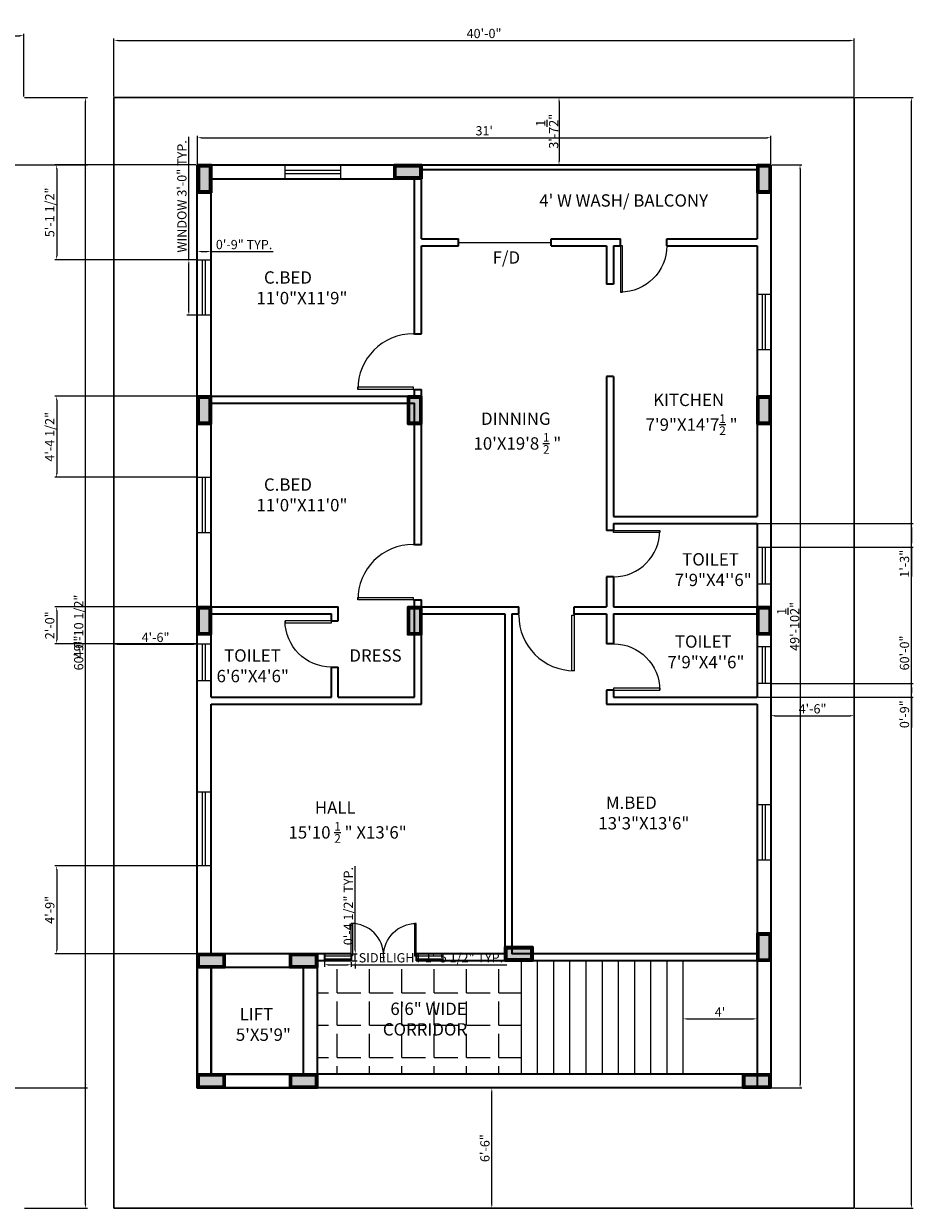
# Model space of a CAD drawing. Units: inches. Extents: x 1678 to 4856, y 4 to 3876.
# Tile 3 of 4: x 2753 to 3330, y 3108 to 3876. Entities that reach past the tile are written whole.
import ezdxf

# ---------------------------------------------------------------- set-up
doc = ezdxf.new("R2010")
doc.units = ezdxf.units.IN
for name, color, linetype, lineweight in [('A-ANNO-TEXT', 7, 'Continuous', 18), ('A-AREA-IDEN', 7, 'Continuous', 18), ('A-FLOR-EVTR', 7, 'Continuous', 35), ('A-FLOR-PATT', 252, 'Continuous', 13), ('COL', 6, 'Continuous', 40), ('compound wall', 7, 'Continuous', 30), ('DIMENSIONS', 6, 'Continuous', 18), ('doors', 2, 'Continuous', 18), ('stairs', 1, 'Continuous', 18), ('walls', 7, 'Continuous', 35), ('windows', 4, 'Continuous', 18)]:
    doc.layers.add(name, color=color, linetype=linetype, lineweight=lineweight)
doc.styles.get("Standard").update_dxf_attribs({"font": 'arial.ttf'})
doc.dimstyles.new('ISO-25', dxfattribs={"dimtxt": 6, "dimasz": 2.5, "dimexe": 1.25, "dimexo": 0.625, "dimtad": 1, "dimdec": 1, "dimlunit": 4, "dimtxsty": 'Standard', "dimcen": 2.5, "dimadec": 0, "dimazin": 0, "dimtfac": 1, "dimtdec": 1, "dimtmove": 0, "dimatfit": 3, "dimfxl": 1, "dimarcsym": 0})

# ---------------------------------------------------------------- blocks, each defined once
blk = doc.blocks.new('*U2')
for p, q in [((0, 0), (0, -6)), ((40, 0), (40, -6))]:
    blk.add_line(p, q)
blk.add_lwpolyline([(0, 0), (0, 40), (1.75, 40), (1.75, 0)], close=True)
blk.add_arc((0, 0), 40, 0, 90)
blk = doc.blocks.new('*D3')
at = {"layer": 'Defpoints', "color": 0, "transparency": 16777216}
for p in [(3180.72, 3232.03), (3228.72, 3232.03), (3228.72, 3231.08)]:
    blk.add_point(p, dxfattribs=at)
at = {"layer": 'DIMENSIONS', "color": 0, "lineweight": -2, "transparency": 16777216}
for p, q in [((3180.72, 3231.4), (3180.72, 3229.83)), ((3183.22, 3231.08), (3226.22, 3231.08)), ((3228.72, 3231.4), (3228.72, 3229.83))]:
    blk.add_line(p, q, dxfattribs=at)
at = {"layer": 'DIMENSIONS', "color": 0, "transparency": 16777216}
for points in [[(3183.22, 3231.5), (3183.22, 3230.67), (3180.72, 3231.08)], [(3226.22, 3231.5), (3226.22, 3230.67), (3228.72, 3231.08)]]:
    blk.add_solid(points, dxfattribs=at)
at = {"layer": 'DIMENSIONS', "color": 0, "transparency": 16777216, "insert": (3204.72, 3234.71), "char_height": 6, "attachment_point": 5}
blk.add_mtext("4'", dxfattribs=at)
blk = doc.blocks.new('*D4')
at = {"layer": 'Defpoints', "color": 0, "transparency": 16777216}
for p in [(3237.72, 3802.31), (2865.95, 3784.66), (3237.72, 3784.66)]:
    blk.add_point(p, dxfattribs=at)
at = {"layer": 'DIMENSIONS', "color": 0, "lineweight": -2, "transparency": 16777216}
for p, q in [((2865.95, 3785.29), (2865.95, 3803.56)), ((2868.45, 3802.31), (3235.22, 3802.31)), ((3237.72, 3785.29), (3237.72, 3803.56))]:
    blk.add_line(p, q, dxfattribs=at)
at = {"layer": 'DIMENSIONS', "color": 0, "transparency": 16777216}
for points in [[(2868.45, 3802.73), (2868.45, 3801.89), (2865.95, 3802.31)], [(3235.22, 3802.73), (3235.22, 3801.89), (3237.72, 3802.31)]]:
    blk.add_solid(points, dxfattribs=at)
at = {"layer": 'DIMENSIONS', "color": 0, "transparency": 16777216, "insert": (3051.84, 3806), "char_height": 6, "attachment_point": 5}
blk.add_mtext("31'", dxfattribs=at)
blk = doc.blocks.new('*D5')
at = {"layer": 'Defpoints', "color": 0, "transparency": 16777216}
for p in [(3083.8, 3828.28), (3083.8, 3784.66), (3100.35, 3784.66)]:
    blk.add_point(p, dxfattribs=at)
at = {"layer": 'DIMENSIONS', "color": 0, "lineweight": -2, "transparency": 16777216}
for p, q in [((3084.43, 3828.28), (3101.6, 3828.28)), ((3100.35, 3825.78), (3100.35, 3787.16)), ((3084.43, 3784.66), (3101.6, 3784.66))]:
    blk.add_line(p, q, dxfattribs=at)
at = {"layer": 'DIMENSIONS', "color": 0, "transparency": 16777216}
for points in [[(3099.93, 3825.78), (3100.76, 3825.78), (3100.35, 3828.28)], [(3099.93, 3787.16), (3100.76, 3787.16), (3100.35, 3784.66)]]:
    blk.add_solid(points, dxfattribs=at)
at = {"layer": 'DIMENSIONS', "color": 0, "transparency": 16777216, "insert": (3092.65, 3806.47), "char_height": 6, "attachment_point": 5, "rotation": 90}
blk.add_mtext('3\'-7{\\H1x;\\S1/2;}"', dxfattribs=at)
blk = doc.blocks.new('*D10')
at = {"layer": 'Defpoints', "color": 0, "transparency": 16777216}
for p in [(2865.72, 3473.89), (2811.72, 3468.28), (2865.72, 3468.28)]:
    blk.add_point(p, dxfattribs=at)
at = {"layer": 'DIMENSIONS', "color": 0, "lineweight": -2, "transparency": 16777216}
for p, q in [((2811.72, 3468.9), (2811.72, 3475.14)), ((2814.22, 3473.89), (2863.22, 3473.89)), ((2865.72, 3468.9), (2865.72, 3475.14))]:
    blk.add_line(p, q, dxfattribs=at)
at = {"layer": 'DIMENSIONS', "color": 0, "transparency": 16777216}
for points in [[(2814.22, 3474.31), (2814.22, 3473.47), (2811.72, 3473.89)], [(2863.22, 3474.31), (2863.22, 3473.47), (2865.72, 3473.89)]]:
    blk.add_solid(points, dxfattribs=at)
at = {"layer": 'DIMENSIONS', "color": 0, "transparency": 16777216, "insert": (2838.72, 3477.58), "char_height": 6, "attachment_point": 5}
blk.add_mtext('4\'-6"', dxfattribs=at)
blk = doc.blocks.new('*D11')
at = {"layer": 'Defpoints', "color": 0, "transparency": 16777216}
for p in [(3237.72, 3429.89), (3291.72, 3429.89), (3291.72, 3427.61)]:
    blk.add_point(p, dxfattribs=at)
at = {"layer": 'DIMENSIONS', "color": 0, "lineweight": -2, "transparency": 16777216}
for p, q in [((3237.72, 3429.27), (3237.72, 3426.36)), ((3240.22, 3427.61), (3289.22, 3427.61)), ((3291.72, 3429.27), (3291.72, 3426.36))]:
    blk.add_line(p, q, dxfattribs=at)
at = {"layer": 'DIMENSIONS', "color": 0, "transparency": 16777216}
for points in [[(3240.22, 3428.02), (3240.22, 3427.19), (3237.72, 3427.61)], [(3289.22, 3428.02), (3289.22, 3427.19), (3291.72, 3427.61)]]:
    blk.add_solid(points, dxfattribs=at)
at = {"layer": 'DIMENSIONS', "color": 0, "transparency": 16777216, "insert": (3264.72, 3431.29), "char_height": 6, "attachment_point": 5}
blk.add_mtext('4\'-6"', dxfattribs=at)
blk = doc.blocks.new('*D12')
at = {"layer": 'Defpoints', "color": 0, "transparency": 16777216}
for p in [(3034.26, 3186.28), (3056.74, 3186.28), (3034.26, 3108.28)]:
    blk.add_point(p, dxfattribs=at)
at = {"layer": 'DIMENSIONS', "color": 0, "lineweight": -2, "transparency": 16777216}
for p, q in [((3034.88, 3186.28), (3057.99, 3186.28)), ((3056.74, 3110.78), (3056.74, 3183.78)), ((3034.88, 3108.28), (3057.99, 3108.28))]:
    blk.add_line(p, q, dxfattribs=at)
at = {"layer": 'DIMENSIONS', "color": 0, "transparency": 16777216}
for points in [[(3056.33, 3183.78), (3057.16, 3183.78), (3056.74, 3186.28)], [(3056.33, 3110.78), (3057.16, 3110.78), (3056.74, 3108.28)]]:
    blk.add_solid(points, dxfattribs=at)
at = {"layer": 'DIMENSIONS', "color": 0, "transparency": 16777216, "insert": (3053.06, 3147.28), "char_height": 6, "attachment_point": 5, "rotation": 90}
blk.add_mtext('6\'-6"', dxfattribs=at)
blk = doc.blocks.new('*D16')
at = {"layer": 'Defpoints', "color": 0, "transparency": 16777216}
for p in [(3237.72, 3784.66), (3237.52, 3186.28), (3256.62, 3186.28)]:
    blk.add_point(p, dxfattribs=at)
at = {"layer": 'DIMENSIONS', "color": 0, "lineweight": -2, "transparency": 16777216}
for p, q in [((3238.34, 3784.66), (3257.87, 3784.66)), ((3256.62, 3782.16), (3256.62, 3188.78)), ((3238.15, 3186.28), (3257.87, 3186.28))]:
    blk.add_line(p, q, dxfattribs=at)
at = {"layer": 'DIMENSIONS', "color": 0, "transparency": 16777216}
for points in [[(3256.2, 3782.16), (3257.03, 3782.16), (3256.62, 3784.66)], [(3256.2, 3188.78), (3257.03, 3188.78), (3256.62, 3186.28)]]:
    blk.add_solid(points, dxfattribs=at)
at = {"layer": 'DIMENSIONS', "color": 0, "transparency": 16777216, "insert": (3248.92, 3485.47), "char_height": 6, "attachment_point": 5, "rotation": 90}
blk.add_mtext('49\'-10{\\H1x;\\S1/2;}"', dxfattribs=at)
blk = doc.blocks.new('COLUMN-9x18')
h = blk.add_hatch(color=256)
h.dxf.hatch_style = 1
h.paths.add_polyline_path([(8, 1), (8, 17), (1, 17), (1, 1)])
for points in [[(9, 18), (9, 0), (0, 0), (0, 18)], [(8, 17), (8, 1), (1, 1), (1, 17)]]:
    blk.add_lwpolyline(points, close=True)
blk = doc.blocks.new('WIN-36')
for p, q in [((3.5, 0), (3.5, 36)), ((5.5, 0), (5.5, 36))]:
    blk.add_line(p, q)
blk.add_lwpolyline([(0, 0), (0, 36), (9, 36), (9, 0)], close=True)
blk = doc.blocks.new('WIN-24')
for p, q in [((3.5, 0), (3.5, 24)), ((5.5, 0), (5.5, 24))]:
    blk.add_line(p, q)
blk.add_lwpolyline([(0, 0), (0, 24), (9, 24), (9, 0)], close=True)
blk = doc.blocks.new('WIN-48')
for p, q in [((3.5, 0), (3.5, 48)), ((5.5, 0), (5.5, 48))]:
    blk.add_line(p, q)
blk.add_lwpolyline([(0, 0), (0, 48), (9, 48), (9, 0)], close=True)
blk = doc.blocks.new('WIN-ENTRY-SIDELIGHT')
for p, q in [((0, 3.25), (17.39, 3.25)), ((0, 1.25), (17.39, 1.25))]:
    blk.add_line(p, q)
blk.add_lwpolyline([(0, 4.5), (17.39, 4.5), (17.39, 0), (0, 0)], close=True)
blk = doc.blocks.new('SITE-PERIMETER-40x60')
for p, q in [((0, 720), (480, 720)), ((0, 0), (0, 720)), ((480, 720), (480, 0)), ((480, 0), (0, 0))]:
    blk.add_line(p, q)
blk = doc.blocks.new('STAIR-FLIGHT-11-TREAD-LINES')
for p, q in [((0, 73.5), (0, 0)), ((10.5, 73.5), (10.5, 0)), ((21, 73.5), (21, 0)), ((31.5, 73.5), (31.5, 0)), ((42, 73.5), (42, 0)), ((52.5, 73.5), (52.5, 0)), ((63, 73.5), (63, 0)), ((73.5, 73.5), (73.5, 0)), ((84, 73.5), (84, 0)), ((94.5, 73.5), (94.5, 0)), ((105, 73.5), (105, 0))]:
    blk.add_line(p, q)
blk = doc.blocks.new('LIFT-SHAFT-60x69')
for p, q in [((9, 9), (9, 78)), ((69, 9), (9, 9))]:
    blk.add_line(p, q)
blk.add_lwpolyline([(78, 87), (78, 87), (0, 87), (0, 0), (78, 0), (78, 82.5)])
blk.add_lwpolyline([(9, 9), (69, 9), (69, 78), (9, 78)], close=True)
blk = doc.blocks.new('*D48')
at = {"layer": 'Defpoints', "color": 0, "transparency": 16777216}
for p in [(2860.32, 3723.16), (2865.72, 3723.16), (2865.72, 3687.16)]:
    blk.add_point(p, dxfattribs=at)
at = {"layer": 'DIMENSIONS', "color": 0, "lineweight": -2, "transparency": 16777216}
for p, q in [((2860.32, 3723.16), (2860.32, 3802.84)), ((2865.09, 3723.16), (2859.07, 3723.16)), ((2860.32, 3689.66), (2860.32, 3720.66)), ((2865.09, 3687.16), (2859.07, 3687.16))]:
    blk.add_line(p, q, dxfattribs=at)
at = {"layer": 'DIMENSIONS', "color": 0, "transparency": 16777216}
for points in [[(2859.9, 3720.66), (2860.73, 3720.66), (2860.32, 3723.16)], [(2859.9, 3689.66), (2860.73, 3689.66), (2860.32, 3687.16)]]:
    blk.add_solid(points, dxfattribs=at)
at = {"layer": 'DIMENSIONS', "color": 0, "transparency": 16777216, "insert": (2856.59, 3764.25), "char_height": 6, "attachment_point": 5, "rotation": 90}
blk.add_mtext('WINDOW 3\'-0" TYP.', dxfattribs=at)
blk = doc.blocks.new('*D49')
at = {"layer": 'Defpoints', "color": 0, "transparency": 16777216}
for p in [(2874.72, 3728.56), (2865.72, 3723.16), (2874.72, 3723.16)]:
    blk.add_point(p, dxfattribs=at)
at = {"layer": 'DIMENSIONS', "color": 0, "lineweight": -2, "transparency": 16777216}
for p, q in [((2865.72, 3723.79), (2865.72, 3729.81)), ((2868.22, 3728.56), (2872.22, 3728.56)), ((2874.72, 3723.79), (2874.72, 3729.81)), ((2874.72, 3728.56), (2915.04, 3728.56))]:
    blk.add_line(p, q, dxfattribs=at)
at = {"layer": 'DIMENSIONS', "color": 0, "transparency": 16777216}
for points in [[(2868.22, 3728.98), (2868.22, 3728.15), (2865.72, 3728.56)], [(2872.22, 3728.98), (2872.22, 3728.15), (2874.72, 3728.56)]]:
    blk.add_solid(points, dxfattribs=at)
at = {"layer": 'DIMENSIONS', "color": 0, "transparency": 16777216, "insert": (2896.13, 3732.25), "char_height": 6, "attachment_point": 5}
blk.add_mtext('0\'-9" TYP.', dxfattribs=at)
blk = doc.blocks.new('*D54')
at = {"layer": 'Defpoints', "color": 0, "transparency": 16777216}
for p in [(2948.22, 3268.78), (2965.61, 3268.78), (2965.61, 3266.17)]:
    blk.add_point(p, dxfattribs=at)
at = {"layer": 'DIMENSIONS', "color": 0, "lineweight": -2, "transparency": 16777216}
for p, q in [((2948.22, 3268.15), (2948.22, 3264.92)), ((2950.72, 3266.17), (2963.11, 3266.17)), ((2965.61, 3268.15), (2965.61, 3264.92)), ((2965.61, 3266.17), (3066.46, 3266.17))]:
    blk.add_line(p, q, dxfattribs=at)
at = {"layer": 'DIMENSIONS', "color": 0, "transparency": 16777216}
for points in [[(2950.72, 3266.59), (2950.72, 3265.75), (2948.22, 3266.17)], [(2963.11, 3266.59), (2963.11, 3265.75), (2965.61, 3266.17)]]:
    blk.add_solid(points, dxfattribs=at)
at = {"layer": 'DIMENSIONS', "color": 0, "transparency": 16777216, "insert": (3017.28, 3269.9), "char_height": 6, "attachment_point": 5}
blk.add_mtext('SIDELIGHT 1\'-5 1/2" TYP.', dxfattribs=at)
blk = doc.blocks.new('*D55')
at = {"layer": 'Defpoints', "color": 0, "transparency": 16777216}
for p in [(2965.61, 3273.28), (2968.22, 3273.28), (2965.61, 3268.78)]:
    blk.add_point(p, dxfattribs=at)
at = {"layer": 'DIMENSIONS', "color": 0, "lineweight": -2, "transparency": 16777216}
for p, q in [((2968.22, 3275.78), (2968.22, 3330.08)), ((2966.23, 3273.28), (2969.47, 3273.28)), ((2968.22, 3268.78), (2968.22, 3273.28)), ((2966.23, 3268.78), (2969.47, 3268.78)), ((2968.22, 3266.28), (2968.22, 3263.78))]:
    blk.add_line(p, q, dxfattribs=at)
at = {"layer": 'DIMENSIONS', "color": 0, "transparency": 16777216}
for points in [[(2967.8, 3275.78), (2968.63, 3275.78), (2968.22, 3273.28)], [(2967.8, 3266.28), (2968.63, 3266.28), (2968.22, 3268.78)]]:
    blk.add_solid(points, dxfattribs=at)
at = {"layer": 'DIMENSIONS', "color": 0, "transparency": 16777216, "insert": (2964.49, 3304.18), "char_height": 6, "attachment_point": 5, "rotation": 90}
blk.add_mtext('0\'-4 1/2" TYP.', dxfattribs=at)
blk = doc.blocks.new('*D57')
at = {"layer": 'Defpoints', "color": 0, "transparency": 16777216}
for p in [(2753.23, 3868.43), (2273.23, 3828.28), (2753.23, 3828.28)]:
    blk.add_point(p, dxfattribs=at)
at = {"layer": 'DIMENSIONS', "color": 0, "lineweight": -2, "transparency": 16777216}
for p, q in [((2273.23, 3828.9), (2273.23, 3869.68)), ((2275.73, 3868.43), (2750.73, 3868.43)), ((2753.23, 3828.9), (2753.23, 3869.68))]:
    blk.add_line(p, q, dxfattribs=at)
at = {"layer": 'DIMENSIONS', "color": 0, "transparency": 16777216}
for points in [[(2275.73, 3868.84), (2275.73, 3868.01), (2273.23, 3868.43)], [(2750.73, 3868.84), (2750.73, 3868.01), (2753.23, 3868.43)]]:
    blk.add_solid(points, dxfattribs=at)
at = {"layer": 'DIMENSIONS', "color": 0, "transparency": 16777216, "insert": (2513.23, 3872.12), "char_height": 6, "attachment_point": 5}
blk.add_mtext('40\'-0"', dxfattribs=at)
blk = doc.blocks.new('*D58')
at = {"layer": 'Defpoints', "color": 0, "transparency": 16777216}
for p in [(2753.23, 3828.28), (2793.38, 3828.28), (2753.23, 3108.28)]:
    blk.add_point(p, dxfattribs=at)
at = {"layer": 'DIMENSIONS', "color": 0, "lineweight": -2, "transparency": 16777216}
for p, q in [((2753.85, 3828.28), (2794.63, 3828.28)), ((2793.38, 3110.78), (2793.38, 3825.78)), ((2753.85, 3108.28), (2794.63, 3108.28))]:
    blk.add_line(p, q, dxfattribs=at)
at = {"layer": 'DIMENSIONS', "color": 0, "transparency": 16777216}
for points in [[(2792.96, 3825.78), (2793.8, 3825.78), (2793.38, 3828.28)], [(2792.96, 3110.78), (2793.8, 3110.78), (2793.38, 3108.28)]]:
    blk.add_solid(points, dxfattribs=at)
at = {"layer": 'DIMENSIONS', "color": 0, "transparency": 16777216, "insert": (2789.69, 3468.28), "char_height": 6, "attachment_point": 5, "rotation": 90}
blk.add_mtext('60\'-0"', dxfattribs=at)
blk = doc.blocks.new('*D59')
at = {"layer": 'Defpoints', "color": 0, "transparency": 16777216}
for p in [(2699.23, 3784.66), (2793.38, 3784.66), (2699.23, 3186.28)]:
    blk.add_point(p, dxfattribs=at)
at = {"layer": 'DIMENSIONS', "color": 0, "lineweight": -2, "transparency": 16777216}
for p, q in [((2699.85, 3784.66), (2794.63, 3784.66)), ((2793.38, 3188.78), (2793.38, 3782.16)), ((2699.85, 3186.28), (2794.63, 3186.28))]:
    blk.add_line(p, q, dxfattribs=at)
at = {"layer": 'DIMENSIONS', "color": 0, "transparency": 16777216}
for points in [[(2792.96, 3782.16), (2793.8, 3782.16), (2793.38, 3784.66)], [(2792.96, 3188.78), (2793.8, 3188.78), (2793.38, 3186.28)]]:
    blk.add_solid(points, dxfattribs=at)
at = {"layer": 'DIMENSIONS', "color": 0, "transparency": 16777216, "insert": (2789.65, 3485.47), "char_height": 6, "attachment_point": 5, "rotation": 90}
blk.add_mtext('49\'-10 1/2"', dxfattribs=at)
blk = doc.blocks.new('*D61')
at = {"layer": 'Defpoints', "color": 0, "transparency": 16777216}
for p in [(3291.72, 3865.38), (2811.72, 3828.28), (3291.72, 3828.28)]:
    blk.add_point(p, dxfattribs=at)
at = {"layer": 'DIMENSIONS', "color": 0, "lineweight": -2, "transparency": 16777216}
for p, q in [((2811.72, 3828.9), (2811.72, 3866.63)), ((2814.22, 3865.38), (3289.22, 3865.38)), ((3291.72, 3828.9), (3291.72, 3866.63))]:
    blk.add_line(p, q, dxfattribs=at)
at = {"layer": 'DIMENSIONS', "color": 0, "transparency": 16777216}
for points in [[(2814.22, 3865.79), (2814.22, 3864.96), (2811.72, 3865.38)], [(3289.22, 3865.79), (3289.22, 3864.96), (3291.72, 3865.38)]]:
    blk.add_solid(points, dxfattribs=at)
at = {"layer": 'DIMENSIONS', "color": 0, "transparency": 16777216, "insert": (3051.72, 3869.07), "char_height": 6, "attachment_point": 5}
blk.add_mtext('40\'-0"', dxfattribs=at)
blk = doc.blocks.new('*D76')
at = {"layer": 'Defpoints', "color": 0, "transparency": 16777216}
for p in [(2865.72, 3784.66), (2774.62, 3723.16), (2865.72, 3723.16)]:
    blk.add_point(p, dxfattribs=at)
at = {"layer": 'DIMENSIONS', "color": 0, "lineweight": -2, "transparency": 16777216}
for p, q in [((2865.09, 3784.66), (2773.37, 3784.66)), ((2774.62, 3782.16), (2774.62, 3725.66)), ((2865.09, 3723.16), (2773.37, 3723.16))]:
    blk.add_line(p, q, dxfattribs=at)
at = {"layer": 'DIMENSIONS', "color": 0, "transparency": 16777216}
for points in [[(2774.2, 3782.16), (2775.03, 3782.16), (2774.62, 3784.66)], [(2774.2, 3725.66), (2775.03, 3725.66), (2774.62, 3723.16)]]:
    blk.add_solid(points, dxfattribs=at)
at = {"layer": 'DIMENSIONS', "color": 0, "transparency": 16777216, "insert": (2770.89, 3753.91), "char_height": 6, "attachment_point": 5, "rotation": 90}
blk.add_mtext('5\'-1 1/2"', dxfattribs=at)
blk = doc.blocks.new('*D77')
at = {"layer": 'Defpoints', "color": 0, "transparency": 16777216}
for p in [(2865.72, 3634.66), (2774.62, 3582.16), (2865.72, 3582.16)]:
    blk.add_point(p, dxfattribs=at)
at = {"layer": 'DIMENSIONS', "color": 0, "lineweight": -2, "transparency": 16777216}
for p, q in [((2865.09, 3634.66), (2773.37, 3634.66)), ((2774.62, 3632.16), (2774.62, 3584.66)), ((2865.09, 3582.16), (2773.37, 3582.16))]:
    blk.add_line(p, q, dxfattribs=at)
at = {"layer": 'DIMENSIONS', "color": 0, "transparency": 16777216}
for points in [[(2774.2, 3632.16), (2775.03, 3632.16), (2774.62, 3634.66)], [(2774.2, 3584.66), (2775.03, 3584.66), (2774.62, 3582.16)]]:
    blk.add_solid(points, dxfattribs=at)
at = {"layer": 'DIMENSIONS', "color": 0, "transparency": 16777216, "insert": (2770.89, 3608.41), "char_height": 6, "attachment_point": 5, "rotation": 90}
blk.add_mtext('4\'-4 1/2"', dxfattribs=at)
blk = doc.blocks.new('*D78')
at = {"layer": 'Defpoints', "color": 0, "transparency": 16777216}
for p in [(2865.72, 3498.16), (2774.62, 3474.26), (2865.72, 3474.26)]:
    blk.add_point(p, dxfattribs=at)
at = {"layer": 'DIMENSIONS', "color": 0, "lineweight": -2, "transparency": 16777216}
for p, q in [((2865.09, 3498.16), (2773.37, 3498.16)), ((2774.62, 3495.66), (2774.62, 3476.76)), ((2865.09, 3474.26), (2773.37, 3474.26))]:
    blk.add_line(p, q, dxfattribs=at)
at = {"layer": 'DIMENSIONS', "color": 0, "transparency": 16777216}
for points in [[(2774.2, 3495.66), (2775.03, 3495.66), (2774.62, 3498.16)], [(2774.2, 3476.76), (2775.03, 3476.76), (2774.62, 3474.26)]]:
    blk.add_solid(points, dxfattribs=at)
at = {"layer": 'DIMENSIONS', "color": 0, "transparency": 16777216, "insert": (2770.93, 3486.21), "char_height": 6, "attachment_point": 5, "rotation": 90}
blk.add_mtext('2\'-0"', dxfattribs=at)
blk = doc.blocks.new('*D79')
at = {"layer": 'Defpoints', "color": 0, "transparency": 16777216}
for p in [(2865.72, 3330.22), (2774.62, 3273.28), (2865.72, 3273.28)]:
    blk.add_point(p, dxfattribs=at)
at = {"layer": 'DIMENSIONS', "color": 0, "lineweight": -2, "transparency": 16777216}
for p, q in [((2865.09, 3330.22), (2773.37, 3330.22)), ((2774.62, 3327.72), (2774.62, 3275.78)), ((2865.09, 3273.28), (2773.37, 3273.28))]:
    blk.add_line(p, q, dxfattribs=at)
at = {"layer": 'DIMENSIONS', "color": 0, "transparency": 16777216}
for points in [[(2774.2, 3327.72), (2775.03, 3327.72), (2774.62, 3330.22)], [(2774.2, 3275.78), (2775.03, 3275.78), (2774.62, 3273.28)]]:
    blk.add_solid(points, dxfattribs=at)
at = {"layer": 'DIMENSIONS', "color": 0, "transparency": 16777216, "insert": (2770.93, 3301.75), "char_height": 6, "attachment_point": 5, "rotation": 90}
blk.add_mtext('4\'-9"', dxfattribs=at)
blk = doc.blocks.new('*D85')
at = {"layer": 'Defpoints', "color": 0, "transparency": 16777216}
for p in [(3228.72, 3552.16), (3237.72, 3536.94), (3328.82, 3536.94)]:
    blk.add_point(p, dxfattribs=at)
at = {"layer": 'DIMENSIONS', "color": 0, "lineweight": -2, "transparency": 16777216}
for p, q in [((3229.34, 3552.16), (3330.07, 3552.16)), ((3328.82, 3549.66), (3328.82, 3539.44)), ((3238.34, 3536.94), (3330.07, 3536.94)), ((3328.82, 3536.94), (3328.82, 3517.81))]:
    blk.add_line(p, q, dxfattribs=at)
at = {"layer": 'DIMENSIONS', "color": 0, "transparency": 16777216}
for points in [[(3328.4, 3549.66), (3329.23, 3549.66), (3328.82, 3552.16)], [(3328.4, 3539.44), (3329.23, 3539.44), (3328.82, 3536.94)]]:
    blk.add_solid(points, dxfattribs=at)
at = {"layer": 'DIMENSIONS', "color": 0, "transparency": 16777216, "insert": (3325.13, 3526.12), "char_height": 6, "attachment_point": 5, "rotation": 90}
blk.add_mtext('1\'-3"', dxfattribs=at)
blk = doc.blocks.new('*D86')
at = {"layer": 'Defpoints', "color": 0, "transparency": 16777216}
for p in [(3237.72, 3448.44), (3228.72, 3439.66), (3328.82, 3439.66)]:
    blk.add_point(p, dxfattribs=at)
at = {"layer": 'DIMENSIONS', "color": 0, "lineweight": -2, "transparency": 16777216}
for p, q in [((3238.34, 3448.44), (3330.07, 3448.44)), ((3328.82, 3445.94), (3328.82, 3442.16)), ((3229.34, 3439.66), (3330.07, 3439.66)), ((3328.82, 3439.66), (3328.82, 3419.96))]:
    blk.add_line(p, q, dxfattribs=at)
at = {"layer": 'DIMENSIONS', "color": 0, "transparency": 16777216}
for points in [[(3328.4, 3445.94), (3329.23, 3445.94), (3328.82, 3448.44)], [(3328.4, 3442.16), (3329.23, 3442.16), (3328.82, 3439.66)]]:
    blk.add_solid(points, dxfattribs=at)
at = {"layer": 'DIMENSIONS', "color": 0, "transparency": 16777216, "insert": (3325.13, 3428.56), "char_height": 6, "attachment_point": 5, "rotation": 90}
blk.add_mtext('0\'-9"', dxfattribs=at)
blk = doc.blocks.new('*D87')
at = {"layer": 'Defpoints', "color": 0, "transparency": 16777216}
for p in [(3291.72, 3828.28), (3328.82, 3828.28), (3291.72, 3108.28)]:
    blk.add_point(p, dxfattribs=at)
at = {"layer": 'DIMENSIONS', "color": 0, "lineweight": -2, "transparency": 16777216}
for p, q in [((3292.34, 3828.28), (3330.07, 3828.28)), ((3328.82, 3110.78), (3328.82, 3825.78)), ((3292.34, 3108.28), (3330.07, 3108.28))]:
    blk.add_line(p, q, dxfattribs=at)
at = {"layer": 'DIMENSIONS', "color": 0, "transparency": 16777216}
for points in [[(3328.4, 3825.78), (3329.23, 3825.78), (3328.82, 3828.28)], [(3328.4, 3110.78), (3329.23, 3110.78), (3328.82, 3108.28)]]:
    blk.add_solid(points, dxfattribs=at)
at = {"layer": 'DIMENSIONS', "color": 0, "transparency": 16777216, "insert": (3325.13, 3468.28), "char_height": 6, "attachment_point": 5, "rotation": 90}
blk.add_mtext('60\'-0"', dxfattribs=at)

msp = doc.modelspace()

# ---------------------------------------------------------------- hatches: boundary and pattern name
at = {"layer": 'A-FLOR-PATT'}
h = msp.add_hatch(dxfattribs=at)
h.set_pattern_fill('ANGLE', color=256, scale=3)
h.set_pattern_definition([(0, (1238.245, 0), (0, 20.955), [15.24, -5.715]), (90, (1238.245, 0), (-20.955, 1e-15), [15.24, -5.715])])
h.paths.add_polyline_path([(3075.72, 3268.78), (2943.72, 3268.78), (2943.72, 3195.28), (3075.72, 3195.28)])

# ---------------------------------------------------------------- linework, layer by layer
at = {"layer": 'doors'}
msp.add_line((3035.22, 3734.41), (3095.22, 3734.41), dxfattribs=at)
at = {"layer": 'walls'}
for p, q in [((2865.72, 3784.66), (3237.72, 3784.66)), ((2865.72, 3186.28), (2865.72, 3784.66)), ((3011.22, 3781.66), (3228.72, 3781.66)), ((3011.22, 3736.66), (3011.22, 3781.66)), ((3228.72, 3781.66), (3228.72, 3736.66)), ((3237.72, 3784.66), (3237.72, 3186.28)), ((2874.72, 3775.66), (3006.72, 3775.66)), ((2874.72, 3634.66), (2874.72, 3775.66)), ((3006.72, 3675.16), (3006.72, 3775.66)), ((3011.22, 3736.66), (3035.22, 3736.66)), ((3011.22, 3732.16), (3035.22, 3732.16)), ((3011.22, 3675.16), (3011.22, 3732.16)), ((3035.22, 3732.16), (3035.22, 3736.66)), ((3095.22, 3732.16), (3095.22, 3736.66)), ((3095.22, 3736.66), (3140.22, 3736.66)), ((3095.22, 3732.16), (3131.22, 3732.16)), ((3131.22, 3732.16), (3131.22, 3707.41)), ((3135.72, 3732.16), (3135.72, 3707.41)), ((3135.72, 3732.16), (3140.22, 3732.16)), ((3140.22, 3732.16), (3140.22, 3736.66)), ((3170.22, 3732.16), (3170.22, 3736.66)), ((3170.22, 3736.66), (3228.72, 3736.66)), ((3170.22, 3732.16), (3228.72, 3732.16)), ((3228.72, 3732.16), (3228.72, 3556.66)), ((3135.72, 3707.41), (3131.22, 3707.41)), ((3006.72, 3675.16), (3011.22, 3675.16)), ((3135.72, 3647.41), (3131.22, 3647.41)), ((3131.22, 3647.41), (3131.22, 3547.66)), ((3135.72, 3647.41), (3135.72, 3556.66)), ((2874.72, 3634.66), (3006.72, 3634.66)), ((3006.72, 3634.66), (3006.72, 3639.16)), ((3006.72, 3639.16), (3011.22, 3639.16)), ((3011.22, 3538.66), (3011.22, 3639.16)), ((2874.72, 3630.16), (3006.72, 3630.16)), ((2874.72, 3498.16), (2874.72, 3630.16)), ((3006.72, 3538.66), (3006.72, 3630.16)), ((3135.72, 3630.16), (3135.72, 3556.66)), ((3135.72, 3556.66), (3228.72, 3556.66)), ((3135.72, 3552.16), (3228.72, 3552.16)), ((3135.72, 3552.16), (3135.72, 3547.66)), ((3228.72, 3552.16), (3228.72, 3498.16)), ((3135.72, 3547.66), (3131.22, 3547.66)), ((3006.72, 3538.66), (3011.22, 3538.66)), ((3135.72, 3517.66), (3131.22, 3517.66)), ((3131.22, 3517.66), (3131.22, 3498.16)), ((3135.72, 3517.66), (3135.72, 3498.16)), ((3006.72, 3498.16), (3006.72, 3502.66)), ((3006.72, 3502.66), (3011.22, 3502.66)), ((3011.22, 3498.16), (3011.22, 3502.66)), ((2874.72, 3498.16), (2957.22, 3498.16)), ((2957.22, 3489.16), (2957.22, 3498.16)), ((3006.72, 3439.66), (3006.72, 3498.16)), ((3011.22, 3498.16), (3074.22, 3498.16)), ((3074.22, 3493.66), (3074.22, 3498.16)), ((3110.22, 3493.66), (3110.22, 3498.16)), ((3110.22, 3498.16), (3131.22, 3498.16)), ((3135.72, 3498.16), (3228.72, 3498.16)), ((2874.72, 3493.66), (2952.72, 3493.66)), ((2874.72, 3439.66), (2874.72, 3493.66)), ((2952.72, 3489.16), (2952.72, 3493.66)), ((2952.72, 3489.16), (2957.22, 3489.16)), ((2957.22, 3489.16), (2957.22, 3489.16)), ((3011.22, 3435.16), (3011.22, 3493.66)), ((3011.22, 3493.66), (3065.22, 3493.66)), ((3065.22, 3493.66), (3065.22, 3273.28)), ((3069.72, 3493.66), (3069.72, 3273.28)), ((3069.72, 3493.66), (3074.22, 3493.66)), ((3110.22, 3493.66), (3131.22, 3493.66)), ((3131.22, 3493.66), (3131.22, 3474.16)), ((3135.72, 3493.66), (3228.72, 3493.66)), ((3135.72, 3493.66), (3135.72, 3474.16)), ((3228.72, 3493.66), (3228.72, 3439.66)), ((3135.72, 3474.16), (3131.22, 3474.16)), ((2952.72, 3439.66), (2952.72, 3459.16)), ((2952.72, 3459.16), (2957.22, 3459.16)), ((2957.22, 3439.66), (2957.22, 3459.16)), ((3135.72, 3444.16), (3131.22, 3444.16)), ((3131.22, 3444.16), (3131.22, 3435.16)), ((3135.72, 3444.16), (3135.72, 3439.66)), ((2874.72, 3439.66), (2952.72, 3439.66)), ((2874.72, 3435.16), (3011.22, 3435.16)), ((2874.72, 3273.28), (2874.72, 3435.16)), ((2957.22, 3439.66), (3006.72, 3439.66)), ((3131.22, 3435.16), (3228.72, 3435.16)), ((3135.72, 3439.66), (3228.72, 3439.66)), ((3228.72, 3435.16), (3228.72, 3268.78)), ((2965.61, 3273.28), (2874.72, 3273.28)), ((2948.22, 3273.28), (2948.22, 3268.78)), ((2948.22, 3273.28), (2948.22, 3268.78)), ((2965.61, 3273.28), (2965.61, 3268.78)), ((3065.22, 3273.28), (3007.61, 3273.28)), ((3007.61, 3273.28), (3007.61, 3268.78)), ((3228.72, 3273.28), (3069.72, 3273.28)), ((2965.61, 3268.78), (2943.72, 3268.78)), ((3228.72, 3268.78), (3007.61, 3268.78)), ((3228.72, 3268.78), (3228.72, 3186.28)), ((3237.72, 3195.28), (2943.72, 3195.28)), ((3237.72, 3186.28), (2865.72, 3186.28))]:
    msp.add_line(p, q, dxfattribs=at)

# ---------------------------------------------------------------- block references
at = {"layer": 'A-FLOR-EVTR'}
msp.add_blockref('LIFT-SHAFT-60x69', (2865.72, 3186.28), dxfattribs=at)
at = {"layer": 'COL'}
for p in [(2865.95, 3766.66), (3228.72, 3766.66), (2865.72, 3616.66), (3002.22, 3616.69), (3228.72, 3616.69), (2865.72, 3480.16), (3002.22, 3480.16), (3228.72, 3480.16), (3228.72, 3268.61)]:
    msp.add_blockref('COLUMN-9x18', p, dxfattribs=at)
for p, rotation in [((3011.35, 3775.66), 90.0000000000118), ((2883.72, 3264.28), 90.00000000000551), ((2943.72, 3264.28), 90.00000000000551), ((3083.27, 3268.78), 90.0000000000076), ((2883.72, 3186.28), 90.00000000000551), ((2943.72, 3186.28), 90.00000000000551), ((3237.52, 3186.28), 90.0000000000076)]:
    msp.add_blockref('COLUMN-9x18', p, dxfattribs=dict(at, rotation=rotation))
at = {"layer": 'compound wall', "rotation": 180}
msp.add_blockref('SITE-PERIMETER-40x60', (3291.72, 3828.28), dxfattribs=at)
at = {"layer": 'doors'}
for p, xscale, yscale, zscale, rotation in [((3140.22, 3732.16), -0.75, 0.75, 0.75, 180), ((3005.82, 3639.16), 0.9, 0.9, 0.9, 89.99999999999999), ((3135.72, 3547.66), 0.75, 0.75, 0.75, 270), ((3005.82, 3502.66), 0.9, 0.9, 0.9, 89.99999999999999), ((3110.22, 3492.76), 0.9, 0.9, 0.9, 180), ((2952.72, 3489.16), -0.75, 0.75, 0.75, 90), ((3135.72, 3444.16), -0.75, 0.75, 0.75, 270)]:
    msp.add_blockref('*U2', p, dxfattribs=dict(at, xscale=xscale, yscale=yscale, zscale=zscale, rotation=rotation))
at = {"layer": 'doors', "yscale": 0.525, "zscale": 0.525}
for p, xscale in [((2965.61, 3271.93), 0.525), ((3007.61, 3271.93), -0.525)]:
    msp.add_blockref('*U2', p, dxfattribs=dict(at, xscale=xscale))
at = {"layer": 'stairs'}
msp.add_blockref('STAIR-FLIGHT-11-TREAD-LINES', (3075.72, 3195.28), dxfattribs=at)
at = {"layer": 'windows', "rotation": 270.0000000000033}
msp.add_blockref('WIN-36', (2922.72, 3784.66), dxfattribs=at)
at = {"layer": 'windows'}
for name, p in [('WIN-36', (2865.72, 3687.16)), ('WIN-36', (3228.72, 3664.81)), ('WIN-36', (2865.72, 3546.16)), ('WIN-24', (3228.72, 3512.94)), ('WIN-24', (2865.72, 3450.26)), ('WIN-24', (3228.72, 3448.44)), ('WIN-48', (2865.72, 3330.22)), ('WIN-36', (3228.72, 3333.97)), ('WIN-ENTRY-SIDELIGHT', (2948.22, 3268.78)), ('WIN-ENTRY-SIDELIGHT', (3007.61, 3268.78))]:
    msp.add_blockref(name, p, dxfattribs=at)

# ---------------------------------------------------------------- texts
at = {"layer": 'A-ANNO-TEXT', "insert": (3057.28, 3728.64), "char_height": 8, "attachment_point": 1}
msp.add_mtext_dynamic_manual_height_columns('F/D', width=15.7651, gutter_width=12.5, heights=[0], dxfattribs=at)
at = {"layer": 'A-AREA-IDEN', "char_height": 8, "attachment_point": 1}
for s, width, insert in [("4' W WASH/ BALCONY", 120.7362, (3087.55, 3765.6)), ('\\pxqj;  C.BED\\P\\pq*;11\'0"X11\'9"', 58.5808, (2904.13, 3715.68)), ('\\A1;  KITCHEN\\P7\'9"X14\'7{\\H0.7x;\\S1/2;} "', 64.7201, (3156.49, 3636.34)), ('\\A1;  DINNING\\P10\'X19\'8 {\\H0.7x;\\S1/2;} "', 64.7201, (3044.89, 3624.15)), ('\\pxqj;  C.BED\\P\\pq*;11\'0"X11\'0"', 58.5808, (2904.13, 3581.44)), ('  TOILET\\P7\'9"X4\'\'6"', 58.5808, (3175.34, 3532.97)), ('  TOILET\\P7\'9"X4\'\'6"', 58.5808, (3170.63, 3479.68)), ('  TOILET\\P6\'6"X4\'6"', 58.5808, (2878.29, 3470.64)), ('  DRESS', 58.5808, (2959.53, 3470.64)), ('\\A1;\\pxqj;       HALL\\P\\pq*;15\'10 {\\H0.7x;\\S1/2;} " X13\'6"', 80.3743, (2924.93, 3372)), ('\\pxqj;  M.BED\\P\\pq*;13\'3"X13\'6"', 58.5808, (3125.84, 3375.22)), ('  6\'6" WIDE\\PCORRIDOR', 58.5808, (2986.1, 3241.61)), (' LIFT\\P5\'X5\'9"', 58.5808, (2890.82, 3238.17))]:
    msp.add_mtext_dynamic_manual_height_columns(s, width=width, gutter_width=12.5, heights=[0], dxfattribs=dict(at, insert=insert))

# ---------------------------------------------------------------- dimensions: what is measured, and where the dimension line sits
at = {"layer": 'DIMENSIONS'}
for base, p1, p2, override, picture, middle in [((2753.23, 3868.43), (2273.23, 3828.28), (2753.23, 3828.28), {"dimdec": 1, "dimlfac": 1, "dimrnd": 0, "dimzin": 1, "dimdsep": 46, "dimlunit": 4, "dimfrac": 2}, '*D57', (2513.23, 3872.12)), ((3291.72, 3865.38), (2811.72, 3828.28), (3291.72, 3828.28), {"dimdec": 1, "dimlfac": 1, "dimrnd": 0, "dimzin": 1, "dimdsep": 46, "dimlunit": 4, "dimfrac": 2}, '*D61', (3051.72, 3869.07)), ((3237.72, 3802.31), (2865.95, 3784.66), (3237.72, 3784.66), {"dimclrd": 0, "dimclre": 0, "dimclrt": 0}, '*D4', (3051.84, 3806)), ((2865.72, 3473.89), (2811.72, 3468.28), (2865.72, 3468.28), {"dimclrd": 0, "dimclre": 0, "dimclrt": 0}, '*D10', (2838.72, 3477.58)), ((3291.72, 3427.61), (3237.72, 3429.89), (3291.72, 3429.89), {"dimclrd": 0, "dimclre": 0, "dimclrt": 0}, '*D11', (3264.72, 3431.29)), ((3228.72, 3231.08), (3180.72, 3232.03), (3228.72, 3232.03), {"dimclrd": 0, "dimclre": 0, "dimclrt": 0}, '*D3', (3204.72, 3234.71))]:
    dim = msp.add_linear_dim(base=base, p1=p1, p2=p2, dimstyle='ISO-25', override=override, dxfattribs=at)
    dim.commit()
    dim.dimension.update_dxf_attribs({"geometry": picture, "text_midpoint": middle})
for base, p1, p2, override, picture, middle in [((2793.38, 3828.28), (2753.23, 3108.28), (2753.23, 3828.28), {"dimdec": 1, "dimlfac": 1, "dimrnd": 0, "dimzin": 1, "dimdsep": 46, "dimlunit": 4, "dimfrac": 2}, '*D58', (2789.69, 3468.28)), ((3100.35, 3784.66), (3083.8, 3828.28), (3083.8, 3784.66), {"dimclrd": 0, "dimclre": 0, "dimclrt": 0}, '*D5', (3092.65, 3806.47)), ((3328.82, 3828.28), (3291.72, 3108.28), (3291.72, 3828.28), {"dimdec": 1, "dimlfac": 1, "dimrnd": 0, "dimzin": 1, "dimdsep": 46, "dimlunit": 4, "dimfrac": 2}, '*D87', (3325.13, 3468.28)), ((2793.38, 3784.66), (2699.23, 3186.28), (2699.23, 3784.66), {"dimdec": 1, "dimlfac": 1, "dimrnd": 0, "dimzin": 1, "dimdsep": 46, "dimlunit": 4, "dimfrac": 2}, '*D59', (2789.65, 3485.47)), ((2774.62, 3723.16), (2865.72, 3784.66), (2865.72, 3723.16), {"dimdec": 1, "dimlfac": 1, "dimrnd": 0, "dimzin": 1, "dimdsep": 46, "dimlunit": 4, "dimfrac": 2}, '*D76', (2770.89, 3753.91)), ((3256.62, 3186.28), (3237.72, 3784.66), (3237.52, 3186.28), {"dimclrd": 0, "dimclre": 0, "dimclrt": 0}, '*D16', (3248.92, 3485.47)), ((2774.62, 3582.16), (2865.72, 3634.66), (2865.72, 3582.16), {"dimdec": 1, "dimlfac": 1, "dimrnd": 0, "dimzin": 1, "dimdsep": 46, "dimlunit": 4, "dimfrac": 2}, '*D77', (2770.89, 3608.41)), ((3328.82, 3536.94), (3228.72, 3552.16), (3237.72, 3536.94), {"dimdec": 1, "dimlfac": 1, "dimrnd": 0, "dimzin": 1, "dimdsep": 46, "dimlunit": 4, "dimfrac": 2}, '*D85', (3325.13, 3526.12)), ((2774.62, 3474.26), (2865.72, 3498.16), (2865.72, 3474.26), {"dimdec": 1, "dimlfac": 1, "dimrnd": 0, "dimzin": 1, "dimdsep": 46, "dimlunit": 4, "dimfrac": 2}, '*D78', (2770.93, 3486.21)), ((3328.82, 3439.66), (3237.72, 3448.44), (3228.72, 3439.66), {"dimdec": 1, "dimlfac": 1, "dimrnd": 0, "dimzin": 1, "dimdsep": 46, "dimlunit": 4, "dimfrac": 2}, '*D86', (3325.13, 3428.56)), ((2774.62, 3273.28), (2865.72, 3330.22), (2865.72, 3273.28), {"dimdec": 1, "dimlfac": 1, "dimrnd": 0, "dimzin": 1, "dimdsep": 46, "dimlunit": 4, "dimfrac": 2}, '*D79', (2770.93, 3301.75)), ((3056.74, 3186.28), (3034.26, 3108.28), (3034.26, 3186.28), {"dimclrd": 0, "dimclre": 0, "dimclrt": 0}, '*D12', (3053.06, 3147.28))]:
    dim = msp.add_linear_dim(base=base, p1=p1, p2=p2, angle=90, dimstyle='ISO-25', override=override, dxfattribs=at)
    dim.commit()
    dim.dimension.update_dxf_attribs({"geometry": picture, "text_midpoint": middle})
for base, p1, p2, text, picture, middle in [((2860.32, 3723.16), (2865.72, 3687.16), (2865.72, 3723.16), 'WINDOW <> TYP.', '*D48', (2856.59, 3764.25)), ((2968.22, 3273.28), (2965.61, 3268.78), (2965.61, 3273.28), '<> TYP.', '*D55', (2964.49, 3304.18))]:
    dim = msp.add_linear_dim(base=base, p1=p1, p2=p2, angle=90, text=text, dimstyle='ISO-25', override={"dimdec": 1, "dimlfac": 1, "dimrnd": 0, "dimzin": 1, "dimdsep": 46, "dimlunit": 4, "dimfrac": 2}, dxfattribs=at)
    dim.commit()
    dim.dimension.update_dxf_attribs({"geometry": picture, "text_midpoint": middle})
for base, p1, p2, text, picture, middle in [((2874.72, 3728.56), (2865.72, 3723.16), (2874.72, 3723.16), '<> TYP.', '*D49', (2896.13, 3732.25)), ((2965.61, 3266.17), (2948.22, 3268.78), (2965.61, 3268.78), 'SIDELIGHT <> TYP.', '*D54', (3017.28, 3269.9))]:
    dim = msp.add_linear_dim(base=base, p1=p1, p2=p2, text=text, dimstyle='ISO-25', override={"dimdec": 1, "dimlfac": 1, "dimrnd": 0, "dimzin": 1, "dimdsep": 46, "dimlunit": 4, "dimfrac": 2}, dxfattribs=at)
    dim.commit()
    dim.dimension.update_dxf_attribs({"geometry": picture, "text_midpoint": middle})

doc.saveas('drawing.dxf')
